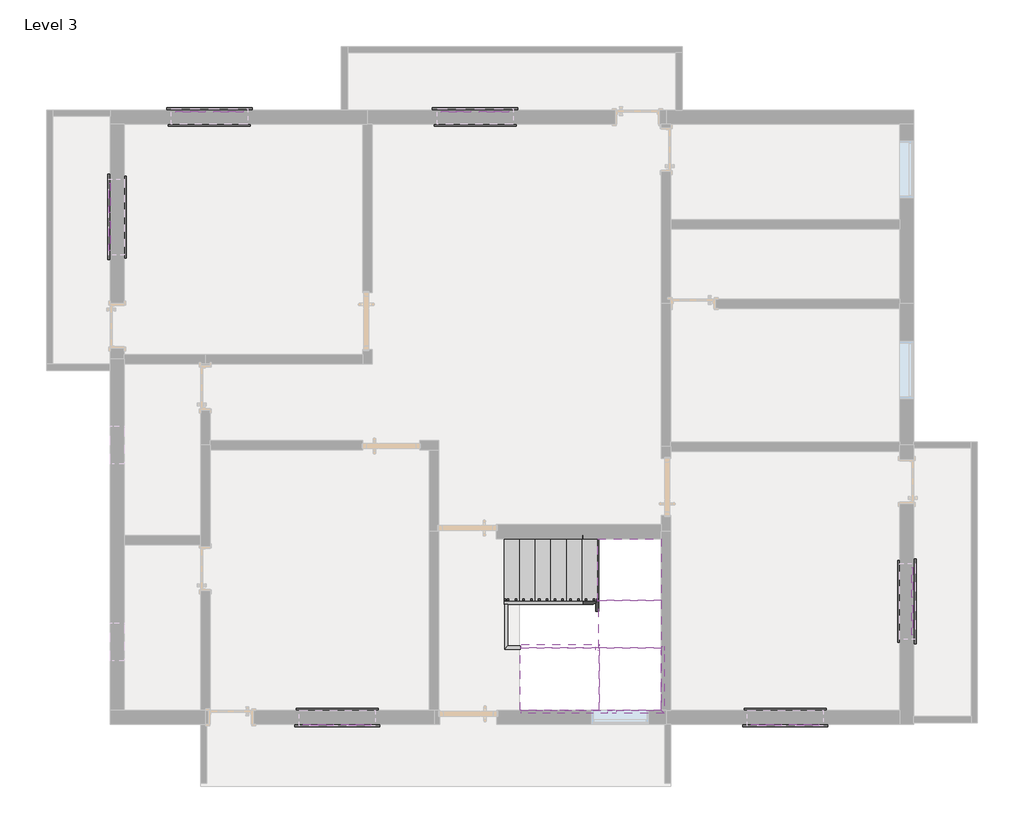
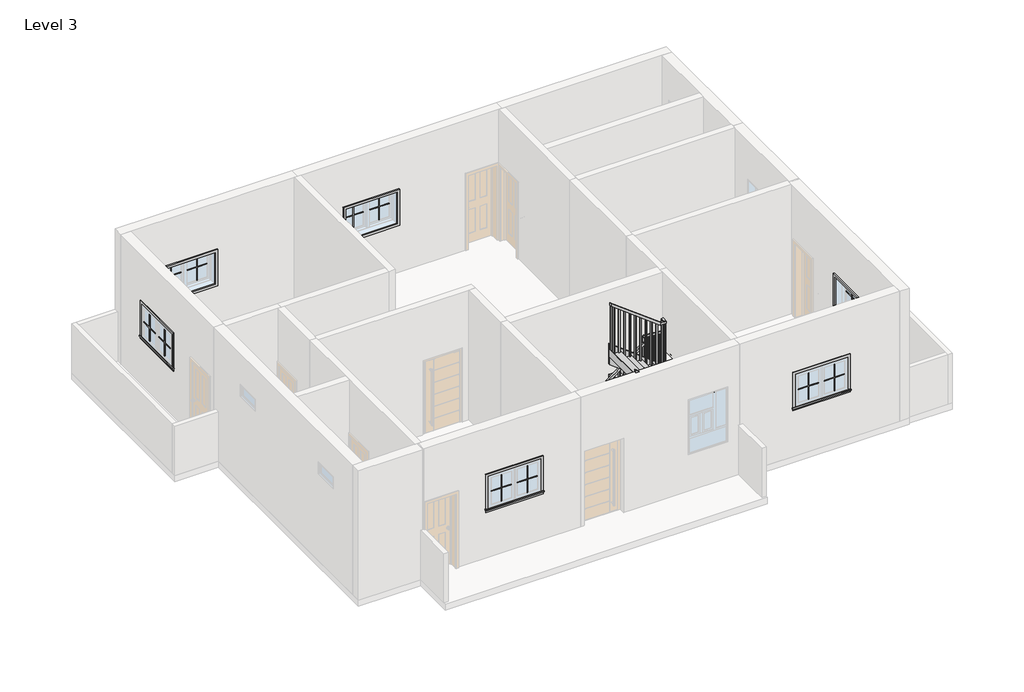
# One storey, part 3 of 3: 24 proxies, 11 members, 3 stair flights, 2 railings, 2 slabs.
"""IFC4 building model written with IfcOpenShell, lengths in millimetres."""

from ifc_helpers import new_model, si_unit, frame, origin, place, context, project, spatial, polyline, outline, extrude, faceted_brep, transform, mapped, element, save
from components import m_muntin_pattern_2x2_m_muntin_pattern_2x2_8d9e5da3, m_muntin_pattern_2x2_m_muntin_pattern_2x2_32a0f80e, m_trim_window_exterior_flat_with_sill_3a557199, m_trim_window_interior_flat_picture_frame_580345df, non_monolithic_landing_7cab632c, non_monolithic_landing_3909d1ad, stair_flight_50mm_tread_13mm_riser_c1773281, stair_flight_50mm_tread_13mm_riser_bd8d9b2e, stair_flight_50mm_tread_13mm_riser_69affff4

model = new_model("IFC4")

# Units and contexts
model_context = context("Model", 3, world=origin())
ifc_project = project(units=[si_unit("LENGTHUNIT", "METRE", prefix="MILLI")], contexts=[model_context])

# Site, building, storey
site = spatial("IfcSite", under=ifc_project)
building = spatial("IfcBuilding", under=site)
storey = spatial("IfcBuildingStorey", under=building, Name="Level 3", Elevation=6400.8)

# Proxies
placement = place(None, origin())
m_muntin_pattern_2x2_m_muntin_pattern_2x2_shape = m_muntin_pattern_2x2_m_muntin_pattern_2x2_8d9e5da3(model_context)
element("IfcBuildingElementProxy", 1, Name="M_Muntin Pattern_2x2 : M_Muntin Pattern_2x2", ObjectType="M_Muntin Pattern_2x2 : M_Muntin Pattern_2x2", at=placement, inside=storey, context=model_context, shape_type="MappedRepresentation", body=[
    mapped(m_muntin_pattern_2x2_m_muntin_pattern_2x2_shape, transform((-14356.7669909, -4470.2368509, 7689.85), x_axis=(-1.0, 0.0, 0.0), y_axis=(0.0, -1.0, 0.0), z_axis=(0.0, 0.0, 1.0))),
])
element("IfcBuildingElementProxy", 2, Name="M_Muntin Pattern_2x2 : M_Muntin Pattern_2x2", ObjectType="M_Muntin Pattern_2x2 : M_Muntin Pattern_2x2", at=placement, inside=storey, context=model_context, shape_type="MappedRepresentation", body=[
    mapped(m_muntin_pattern_2x2_m_muntin_pattern_2x2_shape, transform((-17007.0919909, 5340.5131491, 7689.85), x_axis=(1.0, 0.0, 0.0), y_axis=(0.0, 1.0, 0.0), z_axis=(0.0, 0.0, 1.0))),
])
element("IfcBuildingElementProxy", 3, Name="M_Muntin Pattern_2x2 : M_Muntin Pattern_2x2", ObjectType="M_Muntin Pattern_2x2 : M_Muntin Pattern_2x2", at=placement, inside=storey, context=model_context, shape_type="MappedRepresentation", body=[
    mapped(m_muntin_pattern_2x2_m_muntin_pattern_2x2_shape, transform((-18281.8544909, 3334.7006491, 7689.85), x_axis=(0.0, 1.0, 0.0), y_axis=(-1.0, 0.0, 0.0), z_axis=(0.0, 0.0, 1.0))),
])
element("IfcBuildingElementProxy", 4, Name="M_Muntin Pattern_2x2 : M_Muntin Pattern_2x2", ObjectType="M_Muntin Pattern_2x2 : M_Muntin Pattern_2x2", at=placement, inside=storey, context=model_context, shape_type="MappedRepresentation", body=[
    mapped(m_muntin_pattern_2x2_m_muntin_pattern_2x2_shape, transform((-12757.3544909, 5340.5131491, 7689.85), x_axis=(1.0, 0.0, 0.0), y_axis=(0.0, 1.0, 0.0), z_axis=(0.0, 0.0, 1.0))),
])
element("IfcBuildingElementProxy", 5, Name="M_Muntin Pattern_2x2 : M_Muntin Pattern_2x2", ObjectType="M_Muntin Pattern_2x2 : M_Muntin Pattern_2x2", at=placement, inside=storey, context=model_context, shape_type="MappedRepresentation", body=[
    mapped(m_muntin_pattern_2x2_m_muntin_pattern_2x2_shape, transform((-5448.5044909, -2207.2493509, 7689.85), x_axis=(0.0, -1.0, 0.0), y_axis=(1.0, 0.0, 0.0), z_axis=(0.0, 0.0, 1.0))),
])
element("IfcBuildingElementProxy", 6, Name="M_Muntin Pattern_2x2 : M_Muntin Pattern_2x2", ObjectType="M_Muntin Pattern_2x2 : M_Muntin Pattern_2x2", at=placement, inside=storey, context=model_context, shape_type="MappedRepresentation", body=[
    mapped(m_muntin_pattern_2x2_m_muntin_pattern_2x2_shape, transform((-7193.1669909, -4470.2368509, 7689.85), x_axis=(-1.0, 0.0, 0.0), y_axis=(0.0, -1.0, 0.0), z_axis=(0.0, 0.0, 1.0))),
])
m_muntin_pattern_2x2_m_muntin_pattern_2x2_2_shape = m_muntin_pattern_2x2_m_muntin_pattern_2x2_32a0f80e(model_context)
element("IfcBuildingElementProxy", 7, Name="M_Muntin Pattern_2x2 : M_Muntin Pattern_2x2", ObjectType="M_Muntin Pattern_2x2 : M_Muntin Pattern_2x2", at=placement, inside=storey, context=model_context, shape_type="MappedRepresentation", body=[
    mapped(m_muntin_pattern_2x2_m_muntin_pattern_2x2_2_shape, transform((-14963.1919909, -4470.2368509, 7689.85), x_axis=(1.0, 0.0, 0.0), y_axis=(0.0, 1.0, 0.0), z_axis=(0.0, 0.0, 1.0))),
])
element("IfcBuildingElementProxy", 8, Name="M_Muntin Pattern_2x2 : M_Muntin Pattern_2x2", ObjectType="M_Muntin Pattern_2x2 : M_Muntin Pattern_2x2", at=placement, inside=storey, context=model_context, shape_type="MappedRepresentation", body=[
    mapped(m_muntin_pattern_2x2_m_muntin_pattern_2x2_2_shape, transform((-16400.6669909, 5340.5131491, 7689.85), x_axis=(-1.0, 0.0, 0.0), y_axis=(0.0, -1.0, 0.0), z_axis=(0.0, 0.0, 1.0))),
])
element("IfcBuildingElementProxy", 9, Name="M_Muntin Pattern_2x2 : M_Muntin Pattern_2x2", ObjectType="M_Muntin Pattern_2x2 : M_Muntin Pattern_2x2", at=placement, inside=storey, context=model_context, shape_type="MappedRepresentation", body=[
    mapped(m_muntin_pattern_2x2_m_muntin_pattern_2x2_2_shape, transform((-18281.8544909, 3941.1256491, 7689.85), x_axis=(0.0, -1.0, 0.0), y_axis=(1.0, 0.0, 0.0), z_axis=(0.0, 0.0, 1.0))),
])
element("IfcBuildingElementProxy", 10, Name="M_Muntin Pattern_2x2 : M_Muntin Pattern_2x2", ObjectType="M_Muntin Pattern_2x2 : M_Muntin Pattern_2x2", at=placement, inside=storey, context=model_context, shape_type="MappedRepresentation", body=[
    mapped(m_muntin_pattern_2x2_m_muntin_pattern_2x2_2_shape, transform((-12150.9294909, 5340.5131491, 7689.85), x_axis=(-1.0, 0.0, 0.0), y_axis=(0.0, -1.0, 0.0), z_axis=(0.0, 0.0, 1.0))),
])
element("IfcBuildingElementProxy", 11, Name="M_Muntin Pattern_2x2 : M_Muntin Pattern_2x2", ObjectType="M_Muntin Pattern_2x2 : M_Muntin Pattern_2x2", at=placement, inside=storey, context=model_context, shape_type="MappedRepresentation", body=[
    mapped(m_muntin_pattern_2x2_m_muntin_pattern_2x2_2_shape, transform((-5448.5044909, -2813.6743509, 7689.85), x_axis=(0.0, 1.0, 0.0), y_axis=(-1.0, 0.0, 0.0), z_axis=(0.0, 0.0, 1.0))),
])
element("IfcBuildingElementProxy", 12, Name="M_Muntin Pattern_2x2 : M_Muntin Pattern_2x2", ObjectType="M_Muntin Pattern_2x2 : M_Muntin Pattern_2x2", at=placement, inside=storey, context=model_context, shape_type="MappedRepresentation", body=[
    mapped(m_muntin_pattern_2x2_m_muntin_pattern_2x2_2_shape, transform((-7799.5919909, -4470.2368509, 7689.85), x_axis=(1.0, 0.0, 0.0), y_axis=(0.0, 1.0, 0.0), z_axis=(0.0, 0.0, 1.0))),
])
m_trim_window_exterior_flat_with_sill_shape = m_trim_window_exterior_flat_with_sill_3a557199(model_context)
element("IfcBuildingElementProxy", 13, Name="M_Trim-Window-Exterior-Flat : with Sill", ObjectType="M_Trim-Window-Exterior-Flat : with Sill", at=placement, inside=storey, context=model_context, shape_type="MappedRepresentation", body=[
    mapped(m_trim_window_exterior_flat_with_sill_shape, transform((-14659.9794909, -4479.7618509, 8420.0), x_axis=(1.0, 0.0, 0.0), y_axis=(0.0, 0.0, 1.0), z_axis=(0.0, -1.0, 0.0))),
])
element("IfcBuildingElementProxy", 14, Name="M_Trim-Window-Exterior-Flat : with Sill", ObjectType="M_Trim-Window-Exterior-Flat : with Sill", at=placement, inside=storey, context=model_context, shape_type="MappedRepresentation", body=[
    mapped(m_trim_window_exterior_flat_with_sill_shape, transform((-16703.8794909, 5350.0381491, 8420.0), x_axis=(-1.0, 0.0, 0.0), y_axis=(0.0, 0.0, 1.0), z_axis=(0.0, 1.0, 0.0))),
])
element("IfcBuildingElementProxy", 15, Name="M_Trim-Window-Exterior-Flat : with Sill", ObjectType="M_Trim-Window-Exterior-Flat : with Sill", at=placement, inside=storey, context=model_context, shape_type="MappedRepresentation", body=[
    mapped(m_trim_window_exterior_flat_with_sill_shape, transform((-18291.3794909, 3637.9131491, 8420.0), x_axis=(0.0, -1.0, 0.0), y_axis=(0.0, 0.0, 1.0), z_axis=(-1.0, 0.0, 0.0))),
])
element("IfcBuildingElementProxy", 16, Name="M_Trim-Window-Exterior-Flat : with Sill", ObjectType="M_Trim-Window-Exterior-Flat : with Sill", at=placement, inside=storey, context=model_context, shape_type="MappedRepresentation", body=[
    mapped(m_trim_window_exterior_flat_with_sill_shape, transform((-12454.1419909, 5350.0381491, 8420.0), x_axis=(-1.0, 0.0, 0.0), y_axis=(0.0, 0.0, 1.0), z_axis=(0.0, 1.0, 0.0))),
])
element("IfcBuildingElementProxy", 17, Name="M_Trim-Window-Exterior-Flat : with Sill", ObjectType="M_Trim-Window-Exterior-Flat : with Sill", at=placement, inside=storey, context=model_context, shape_type="MappedRepresentation", body=[
    mapped(m_trim_window_exterior_flat_with_sill_shape, transform((-5438.9794909, -2510.4618509, 8420.0), x_axis=(0.0, 1.0, 0.0), y_axis=(0.0, 0.0, 1.0), z_axis=(1.0, 0.0, 0.0))),
])
element("IfcBuildingElementProxy", 18, Name="M_Trim-Window-Exterior-Flat : with Sill", ObjectType="M_Trim-Window-Exterior-Flat : with Sill", at=placement, inside=storey, context=model_context, shape_type="MappedRepresentation", body=[
    mapped(m_trim_window_exterior_flat_with_sill_shape, transform((-7496.3794909, -4479.7618509, 8420.0), x_axis=(1.0, 0.0, 0.0), y_axis=(0.0, 0.0, 1.0), z_axis=(0.0, -1.0, 0.0))),
])
m_trim_window_interior_flat_picture_frame_shape = m_trim_window_interior_flat_picture_frame_580345df(model_context)
element("IfcBuildingElementProxy", 19, Name="M_Trim-Window-Interior-Flat : Picture Frame", ObjectType="M_Trim-Window-Interior-Flat : Picture Frame", at=placement, inside=storey, context=model_context, shape_type="MappedRepresentation", body=[
    mapped(m_trim_window_interior_flat_picture_frame_shape, transform((-14659.9794909, -4251.1618509, 8420.0), x_axis=(-1.0, 0.0, 0.0), y_axis=(0.0, 0.0, 1.0), z_axis=(0.0, 1.0, 0.0))),
])
element("IfcBuildingElementProxy", 20, Name="M_Trim-Window-Interior-Flat : Picture Frame", ObjectType="M_Trim-Window-Interior-Flat : Picture Frame", at=placement, inside=storey, context=model_context, shape_type="MappedRepresentation", body=[
    mapped(m_trim_window_interior_flat_picture_frame_shape, transform((-16703.8794909, 5121.4381491, 8420.0), x_axis=(1.0, 0.0, 0.0), y_axis=(0.0, 0.0, 1.0), z_axis=(0.0, -1.0, 0.0))),
])
element("IfcBuildingElementProxy", 21, Name="M_Trim-Window-Interior-Flat : Picture Frame", ObjectType="M_Trim-Window-Interior-Flat : Picture Frame", at=placement, inside=storey, context=model_context, shape_type="MappedRepresentation", body=[
    mapped(m_trim_window_interior_flat_picture_frame_shape, transform((-18062.7794909, 3637.9131491, 8420.0), x_axis=(0.0, 1.0, 0.0), y_axis=(0.0, 0.0, 1.0), z_axis=(1.0, 0.0, 0.0))),
])
element("IfcBuildingElementProxy", 22, Name="M_Trim-Window-Interior-Flat : Picture Frame", ObjectType="M_Trim-Window-Interior-Flat : Picture Frame", at=placement, inside=storey, context=model_context, shape_type="MappedRepresentation", body=[
    mapped(m_trim_window_interior_flat_picture_frame_shape, transform((-12454.1419909, 5121.4381491, 8420.0), x_axis=(1.0, 0.0, 0.0), y_axis=(0.0, 0.0, 1.0), z_axis=(0.0, -1.0, 0.0))),
])
element("IfcBuildingElementProxy", 23, Name="M_Trim-Window-Interior-Flat : Picture Frame", ObjectType="M_Trim-Window-Interior-Flat : Picture Frame", at=placement, inside=storey, context=model_context, shape_type="MappedRepresentation", body=[
    mapped(m_trim_window_interior_flat_picture_frame_shape, transform((-5667.5794909, -2510.4618509, 8420.0), x_axis=(0.0, -1.0, 0.0), y_axis=(0.0, 0.0, 1.0), z_axis=(-1.0, 0.0, 0.0))),
])
element("IfcBuildingElementProxy", 24, Name="M_Trim-Window-Interior-Flat : Picture Frame", ObjectType="M_Trim-Window-Interior-Flat : Picture Frame", at=placement, inside=storey, context=model_context, shape_type="MappedRepresentation", body=[
    mapped(m_trim_window_interior_flat_picture_frame_shape, transform((-7496.3794909, -4251.1618509, 8420.0), x_axis=(-1.0, 0.0, 0.0), y_axis=(0.0, 0.0, 1.0), z_axis=(0.0, 1.0, 0.0))),
])

# Members
element("IfcMember", 25, ObjectType="Stringer - 50mm Width", at=placement, inside=storey, context=model_context, shape_type="SweptSolid", body=[
    extrude(outline(polyline([(6654.3429417, -11992.1794909), (6400.8, -11992.1794909), (6400.8, -11663.9259909), (7368.6117647, -10378.7116427), (7768.6117647, -10512.4761733), (6654.3429417, -11992.1794909)])), frame((0.0, -1507.9618509, 0.0), z_axis=(0.0, 1.0, 0.0), x_axis=(0.0, 0.0, 1.0)), (0.0, 0.0, 1.0), 50.0),
])
element("IfcMember", 26, ObjectType="Stringer - 50mm Width", at=placement, inside=storey, context=model_context, shape_type="Brep", body=[
    faceted_brep([(-11992.1794909, -2557.9876321, 6400.8), (-11992.1794909, -2507.9876321, 6400.8), (-11663.9259909, -2507.9876321, 6400.8), (-11663.9259909, -2557.9876321, 6400.8), (-11992.1794909, -2557.9876321, 6654.3429417), (-10569.4898929, -2557.9876321, 7224.949009), (-10569.4898929, -2557.9876321, 7725.6784216), (-10492.1794909, -2507.9876321, 7283.1664703), (-10492.1794909, -2507.9876321, 7768.6117647), (-10512.4761733, -2521.1143795, 7768.6117647), (-11992.1794909, -2507.9876321, 6654.3429417), (-10512.4761733, -2507.9876321, 7768.6117647)], [[[0, 1, 2, 3]], [[4, 0, 3, 5, 6]], [[6, 5, 7, 8, 9]], [[2, 7, 5, 3]], [[1, 10, 11, 8, 7, 2]], [[11, 9, 8]], [[10, 4, 6, 9, 11]], [[4, 10, 1, 0]]]),
])
element("IfcMember", 27, ObjectType="Stringer - 50mm Width", at=placement, inside=storey, context=model_context, shape_type="SweptSolid", body=[
    extrude(outline(polyline([(-2228.2651685, 7768.6117647), (-2362.029699, 7368.6117647), (-3362.029699, 8121.6470588), (-3228.2651685, 8521.6470588), (-2228.2651685, 7768.6117647)])), frame((-9477.5794909, 0.0, 0.0), z_axis=(1.0, 0.0, 0.0), x_axis=(0.0, 1.0, 0.0)), (0.0, 0.0, 1.0), 50.0),
])
element("IfcMember", 28, ObjectType="Stringer - 50mm Width", at=placement, inside=storey, context=model_context, shape_type="Brep", body=[
    faceted_brep([(-10527.6052721, -3234.9066499, 8521.6470588), (-10527.6052721, -3234.9066499, 8025.9189161), (-10477.6052721, -3248.5618509, 8036.2017644), (-10477.6052721, -3248.5618509, 8521.6470588), (-10477.6052721, -3228.2651685, 8521.6470588), (-10527.6052721, -3228.2651685, 8521.6470588), (-10477.6052721, -2498.5618509, 7972.1547064), (-10527.6052721, -2530.8990259, 7996.5057405), (-10477.6052721, -2498.5618509, 7471.4252938), (-10527.6052721, -2530.8990259, 7495.7763279)], [[[0, 1, 2, 3]], [[4, 5, 0, 3]], [[6, 7, 5, 4]], [[7, 6, 8, 9]], [[7, 9, 1, 0, 5]], [[8, 6, 4, 3, 2]], [[9, 8, 2, 1]]]),
])
element("IfcMember", 29, ObjectType="Stringer - 50mm Width", at=placement, inside=storey, context=model_context, shape_type="Brep", body=[
    faceted_brep([(-9477.5794909, -2228.2651685, 7768.6117647), (-9427.5794909, -2228.2651685, 7768.6117647), (-9427.5794909, -1457.9618509, 7768.6117647), (-9477.5794909, -1507.9618509, 7768.6117647), (-9477.5794909, -2362.029699, 7368.6117647), (-9477.5794909, -1507.9618509, 7368.6117647), (-9427.5794909, -2362.029699, 7368.6117647), (-9427.5794909, -1457.9618509, 7368.6117647)], [[[0, 1, 2, 3]], [[4, 0, 3, 5]], [[6, 4, 5, 7]], [[1, 6, 7, 2]], [[1, 0, 4, 6]], [[2, 7, 5, 3]]]),
])
element("IfcMember", 30, ObjectType="Stringer - 50mm Width", at=placement, inside=storey, context=model_context, shape_type="Brep", body=[
    faceted_brep([(-9477.5794909, -1507.9618509, 7768.6117647), (-9427.5794909, -1457.9618509, 7768.6117647), (-10512.4761733, -1457.9618509, 7768.6117647), (-10512.4761733, -1507.9618509, 7768.6117647), (-9477.5794909, -1507.9618509, 7368.6117647), (-10378.7116427, -1507.9618509, 7368.6117647), (-9427.5794909, -1457.9618509, 7368.6117647), (-10378.7116427, -1457.9618509, 7368.6117647)], [[[0, 1, 2, 3]], [[4, 0, 3, 5]], [[6, 4, 5, 7]], [[1, 6, 7, 2]], [[1, 0, 4, 6]], [[2, 7, 5, 3]]]),
])
element("IfcMember", 31, ObjectType="Stringer - 50mm Width", at=placement, inside=storey, context=model_context, shape_type="SweptSolid", body=[
    extrude(outline(polyline([(8121.6470588, -10331.6473391), (8521.6470588, -10197.8828085), (9666.4841182, -11718.1794909), (9165.7547056, -11718.1794909), (8121.6470588, -10331.6473391)])), frame((0.0, -4301.1618509, 0.0), z_axis=(0.0, 1.0, 0.0), x_axis=(0.0, 0.0, 1.0)), (0.0, 0.0, 1.0), 50.0),
])
element("IfcMember", 32, ObjectType="Stringer - 50mm Width", at=placement, inside=storey, context=model_context, shape_type="SweptSolid", body=[
    extrude(outline(polyline([(8224.4605879, -10468.1794909), (8725.1900005, -10468.1794909), (9666.4841182, -11718.1794909), (9165.7547056, -11718.1794909), (8224.4605879, -10468.1794909)])), frame((0.0, -3251.1360696, 0.0), z_axis=(0.0, 1.0, 0.0), x_axis=(0.0, 0.0, 1.0)), (0.0, 0.0, 1.0), 50.0),
])
element("IfcMember", 33, ObjectType="Stringer - 50mm Width", at=placement, inside=storey, context=model_context, shape_type="Brep", body=[
    faceted_brep([(-10197.8828085, -4251.1618509, 8521.6470588), (-10197.8828085, -4301.1618509, 8521.6470588), (-9427.5794909, -4301.1618509, 8521.6470588), (-9477.5794909, -4251.1618509, 8521.6470588), (-10331.6473391, -4251.1618509, 8121.6470588), (-9477.5794909, -4251.1618509, 8121.6470588), (-10331.6473391, -4301.1618509, 8121.6470588), (-9427.5794909, -4301.1618509, 8121.6470588)], [[[0, 1, 2, 3]], [[4, 0, 3, 5]], [[6, 4, 5, 7]], [[1, 6, 7, 2]], [[1, 0, 4, 6]], [[2, 7, 5, 3]]]),
])
element("IfcMember", 34, ObjectType="Stringer - 50mm Width", at=placement, inside=storey, context=model_context, shape_type="Brep", body=[
    faceted_brep([(-9477.5794909, -4251.1618509, 8521.6470588), (-9427.5794909, -4301.1618509, 8521.6470588), (-9427.5794909, -3228.2651685, 8521.6470588), (-9477.5794909, -3228.2651685, 8521.6470588), (-9477.5794909, -4251.1618509, 8121.6470588), (-9477.5794909, -3362.029699, 8121.6470588), (-9427.5794909, -4301.1618509, 8121.6470588), (-9427.5794909, -3362.029699, 8121.6470588)], [[[0, 1, 2, 3]], [[4, 0, 3, 5]], [[6, 4, 5, 7]], [[1, 6, 7, 2]], [[1, 0, 4, 6]], [[2, 7, 5, 3]]]),
])
element("IfcMember", 35, ObjectType="Stringer - 50mm Width", at=placement, inside=storey, context=model_context, shape_type="SweptSolid", body=[
    extrude(outline(polyline([(-10527.6052721, -3286.7377652), (-10527.6052721, -3234.9066499), (-10468.1794909, -3251.1360696), (-10468.1794909, -3302.9671849), (-10527.6052721, -3286.7377652)])), frame((0.0, 0.0, 8121.6470588), z_axis=(0.0, 0.0, 1.0), x_axis=(1.0, 0.0, 0.0)), (0.0, 0.0, 1.0), 400.0),
])

# Railings
element("IfcRailing", 36, ObjectType="1100mm", at=placement, inside=storey, context=model_context, shape_type="SolidModel", body=[
    faceted_brep([(-11992.1794909, -2457.5876321, 7689.0588235), (-11992.1794909, -2457.5876321, 7626.467647), (-11992.1794909, -2507.5876321, 7626.467647), (-11992.1794909, -2507.5876321, 7689.0588235), (-10506.1686883, -2457.5876321, 8808.0774053), (-10493.1861187, -2507.5876321, 8817.8537384), (-10475.1839648, -2507.5876321, 8768.8188191), (-10488.1665344, -2457.5876321, 8759.042486)], [[[0, 1, 2, 3]], [[4, 5, 6, 7]], [[1, 0, 4, 7]], [[2, 1, 7, 6]], [[3, 2, 6, 5]], [[0, 3, 5, 4]]]),
    faceted_brep([(-10507.8033465, -2458.0701724, 8818.6117647), (-10492.6871017, -2448.2938394, 8768.6117647), (-10476.4352157, -2497.3287587, 8768.6117647), (-10491.5514605, -2507.1050918, 8818.6117647), (-10486.7741604, -2444.469683, 8818.6117647), (-10459.6209288, -2486.4542279, 8818.6117647), (-10417.6363839, -2459.3009964, 8768.6117647), (-10444.7896154, -2417.3164514, 8768.6117647)], [[[0, 1, 2, 3]], [[4, 5, 6, 7]], [[1, 0, 4, 7]], [[2, 1, 7, 6]], [[3, 2, 6, 5]], [[0, 3, 5, 4]]]),
    faceted_brep([(-10486.7741604, -2444.469683, 8818.6117647), (-10444.7896154, -2417.3164514, 8768.6117647), (-10417.6363839, -2459.3009964, 8768.6117647), (-10459.6209288, -2486.4542279, 8818.6117647), (-10486.7741604, -2444.469683, 8944.124782), (-10459.6209288, -2486.4542279, 8923.1833848), (-10417.6363839, -2459.3009964, 8936.7270973), (-10444.7896154, -2417.3164514, 8957.6684945)], [[[0, 1, 2, 3]], [[4, 5, 6, 7]], [[1, 0, 4, 7]], [[2, 1, 7, 6]], [[3, 2, 6, 5]], [[0, 3, 5, 4]]]),
    faceted_brep([(-10427.2052721, -2426.8853397, 8952.8956456), (-10427.2052721, -2476.8853397, 8927.9562337), (-10477.2052721, -2476.8853397, 8927.9562337), (-10477.2052721, -2426.8853397, 8952.8956456), (-10427.2052721, -3176.5360696, 9517.4091035), (-10427.2052721, -3226.5360696, 9492.4696916), (-10477.2052721, -3226.5360696, 9492.4696916), (-10477.2052721, -3176.5360696, 9517.4091035), (-10427.2052721, -3176.5360696, 9823.1802613), (-10427.2052721, -3226.5360696, 9773.1802613), (-10477.2052721, -3226.5360696, 9773.1802613), (-10477.2052721, -3176.5360696, 9823.1802613), (-10427.2052721, -3301.5360696, 9823.1802613), (-10427.2052721, -3301.5360696, 9773.1802613), (-10477.2052721, -3251.5360696, 9773.1802613), (-10477.2052721, -3251.5360696, 9823.1802613), (-10552.2052721, -3301.5360696, 9823.1802613), (-10568.9258385, -3301.5360696, 9773.1802613), (-10568.9258385, -3251.5360696, 9773.1802613), (-10552.2052721, -3251.5360696, 9823.1802613), (-11718.1794909, -3301.5360696, 10701.2), (-11718.1794909, -3251.5360696, 10701.2), (-11718.1794909, -3251.5360696, 10638.6088234), (-11718.1794909, -3301.5360696, 10638.6088234)], [[[0, 1, 2, 3]], [[1, 0, 4, 5]], [[2, 1, 5, 6]], [[3, 2, 6, 7]], [[0, 3, 7, 4]], [[5, 4, 8, 9]], [[6, 5, 9, 10]], [[7, 6, 10, 11]], [[4, 7, 11, 8]], [[9, 8, 12, 13]], [[10, 9, 13, 14]], [[11, 10, 14, 15]], [[8, 11, 15, 12]], [[13, 12, 16, 17]], [[14, 13, 17, 18]], [[15, 14, 18, 19]], [[12, 15, 19, 16]], [[20, 21, 22, 23]], [[17, 16, 20, 23]], [[18, 17, 23, 22]], [[19, 18, 22, 21]], [[16, 19, 21, 20]]]),
    extrude(outline(polyline([(9412.9411765, -11627.2052721), (10570.1020258, -11627.2052721), (10588.9279082, -11652.2052721), (9412.9411765, -11652.2052721), (9412.9411765, -11627.2052721)])), frame((0.0, -3289.0360696, 0.0), z_axis=(0.0, 1.0, 0.0), x_axis=(0.0, 0.0, 1.0)), (0.0, 0.0, 1.0), 25.0),
    extrude(outline(polyline([(9412.9411765, -11502.2052721), (10475.9726141, -11502.2052721), (10494.7984964, -11527.2052721), (9412.9411765, -11527.2052721), (9412.9411765, -11502.2052721)])), frame((0.0, -3289.0360696, 0.0), z_axis=(0.0, 1.0, 0.0), x_axis=(0.0, 0.0, 1.0)), (0.0, 0.0, 1.0), 25.0),
    extrude(outline(polyline([(9224.6823529, -11377.2052721), (10381.8432023, -11377.2052721), (10400.6690847, -11402.2052721), (9224.6823529, -11402.2052721), (9224.6823529, -11377.2052721)])), frame((0.0, -3289.0360696, 0.0), z_axis=(0.0, 1.0, 0.0), x_axis=(0.0, 0.0, 1.0)), (0.0, 0.0, 1.0), 25.0),
    extrude(outline(polyline([(9224.6823529, -11252.2052721), (10287.7137906, -11252.2052721), (10306.5396729, -11277.2052721), (9224.6823529, -11277.2052721), (9224.6823529, -11252.2052721)])), frame((0.0, -3289.0360696, 0.0), z_axis=(0.0, 1.0, 0.0), x_axis=(0.0, 0.0, 1.0)), (0.0, 0.0, 1.0), 25.0),
    extrude(outline(polyline([(9036.4235294, -11127.2052721), (10193.5843788, -11127.2052721), (10212.4102611, -11152.2052721), (9036.4235294, -11152.2052721), (9036.4235294, -11127.2052721)])), frame((0.0, -3289.0360696, 0.0), z_axis=(0.0, 1.0, 0.0), x_axis=(0.0, 0.0, 1.0)), (0.0, 0.0, 1.0), 25.0),
    extrude(outline(polyline([(9036.4235294, -11002.2052721), (10099.454967, -11002.2052721), (10118.2808494, -11027.2052721), (9036.4235294, -11027.2052721), (9036.4235294, -11002.2052721)])), frame((0.0, -3289.0360696, 0.0), z_axis=(0.0, 1.0, 0.0), x_axis=(0.0, 0.0, 1.0)), (0.0, 0.0, 1.0), 25.0),
    extrude(outline(polyline([(8848.1647059, -10877.2052721), (10005.3255553, -10877.2052721), (10024.1514376, -10902.2052721), (8848.1647059, -10902.2052721), (8848.1647059, -10877.2052721)])), frame((0.0, -3289.0360696, 0.0), z_axis=(0.0, 1.0, 0.0), x_axis=(0.0, 0.0, 1.0)), (0.0, 0.0, 1.0), 25.0),
    extrude(outline(polyline([(8848.1647059, -10752.2052721), (9911.1961435, -10752.2052721), (9930.0220258, -10777.2052721), (8848.1647059, -10777.2052721), (8848.1647059, -10752.2052721)])), frame((0.0, -3289.0360696, 0.0), z_axis=(0.0, 1.0, 0.0), x_axis=(0.0, 0.0, 1.0)), (0.0, 0.0, 1.0), 25.0),
    extrude(outline(polyline([(8659.9058824, -10627.2052721), (9817.0667317, -10627.2052721), (9835.8926141, -10652.2052721), (8659.9058824, -10652.2052721), (8659.9058824, -10627.2052721)])), frame((0.0, -3289.0360696, 0.0), z_axis=(0.0, 1.0, 0.0), x_axis=(0.0, 0.0, 1.0)), (0.0, 0.0, 1.0), 25.0),
    extrude(outline(polyline([(-10502.2052721, -3264.0360696), (-10502.2052721, -3289.0360696), (-10527.2052721, -3289.0360696), (-10527.2052721, -3264.0360696), (-10502.2052721, -3264.0360696)])), frame((0.0, 0.0, 8659.9058824), z_axis=(0.0, 0.0, 1.0), x_axis=(1.0, 0.0, 0.0)), (0.0, 0.0, 1.0), 1113.2743789),
    extrude(outline(polyline([(-10464.7052721, -3251.8853397), (-10439.7052721, -3251.8853397), (-10439.7052721, -3276.8853397), (-10464.7052721, -3276.8853397), (-10464.7052721, -3251.8853397)])), frame((0.0, 0.0, 8471.6470588), z_axis=(0.0, 0.0, 1.0), x_axis=(1.0, 0.0, 0.0)), (0.0, 0.0, 1.0), 1301.5332024),
    extrude(outline(polyline([(-3126.8853397, 9417.4291749), (-3126.8853397, 8283.3882353), (-3151.8853397, 8283.3882353), (-3151.8853397, 9436.2550572), (-3126.8853397, 9417.4291749)])), frame((-10464.7052721, 0.0, 0.0), z_axis=(1.0, 0.0, 0.0), x_axis=(0.0, 1.0, 0.0)), (0.0, 0.0, 1.0), 25.0),
    extrude(outline(polyline([(-3001.8853397, 9323.2997631), (-3001.8853397, 8283.3882353), (-3026.8853397, 8283.3882353), (-3026.8853397, 9342.1256455), (-3001.8853397, 9323.2997631)])), frame((-10464.7052721, 0.0, 0.0), z_axis=(1.0, 0.0, 0.0), x_axis=(0.0, 1.0, 0.0)), (0.0, 0.0, 1.0), 25.0),
    extrude(outline(polyline([(-2876.8853397, 9229.1703513), (-2876.8853397, 8095.1294118), (-2901.8853397, 8095.1294118), (-2901.8853397, 9247.9962337), (-2876.8853397, 9229.1703513)])), frame((-10464.7052721, 0.0, 0.0), z_axis=(1.0, 0.0, 0.0), x_axis=(0.0, 1.0, 0.0)), (0.0, 0.0, 1.0), 25.0),
    extrude(outline(polyline([(-2751.8853397, 9135.0409396), (-2751.8853397, 8095.1294118), (-2776.8853397, 8095.1294118), (-2776.8853397, 9153.8668219), (-2751.8853397, 9135.0409396)])), frame((-10464.7052721, 0.0, 0.0), z_axis=(1.0, 0.0, 0.0), x_axis=(0.0, 1.0, 0.0)), (0.0, 0.0, 1.0), 25.0),
    extrude(outline(polyline([(-2626.8853397, 9040.9115278), (-2626.8853397, 7906.8705882), (-2651.8853397, 7906.8705882), (-2651.8853397, 9059.7374102), (-2626.8853397, 9040.9115278)])), frame((-10464.7052721, 0.0, 0.0), z_axis=(1.0, 0.0, 0.0), x_axis=(0.0, 1.0, 0.0)), (0.0, 0.0, 1.0), 25.0),
    extrude(outline(polyline([(-2501.8853397, 8946.782116), (-2501.8853397, 7906.8705882), (-2526.8853397, 7906.8705882), (-2526.8853397, 8965.6079984), (-2501.8853397, 8946.782116)])), frame((-10464.7052721, 0.0, 0.0), z_axis=(1.0, 0.0, 0.0), x_axis=(0.0, 1.0, 0.0)), (0.0, 0.0, 1.0), 25.0),
    extrude(outline(polyline([(8699.5429411, -10567.1794909), (7530.3529412, -10567.1794909), (7530.3529412, -10542.1794909), (8718.3688234, -10542.1794909), (8699.5429411, -10567.1794909)])), frame((0.0, -2495.0876321, 0.0), z_axis=(0.0, 1.0, 0.0), x_axis=(0.0, 0.0, 1.0)), (0.0, 0.0, 1.0), 25.0),
    extrude(outline(polyline([(8605.4135293, -10692.1794909), (7530.3529412, -10692.1794909), (7530.3529412, -10667.1794909), (8624.2394117, -10667.1794909), (8605.4135293, -10692.1794909)])), frame((0.0, -2495.0876321, 0.0), z_axis=(0.0, 1.0, 0.0), x_axis=(0.0, 0.0, 1.0)), (0.0, 0.0, 1.0), 25.0),
    extrude(outline(polyline([(8511.2841175, -10817.1794909), (7342.0941176, -10817.1794909), (7342.0941176, -10792.1794909), (8530.1099999, -10792.1794909), (8511.2841175, -10817.1794909)])), frame((0.0, -2495.0876321, 0.0), z_axis=(0.0, 1.0, 0.0), x_axis=(0.0, 0.0, 1.0)), (0.0, 0.0, 1.0), 25.0),
    extrude(outline(polyline([(8417.1547058, -10942.1794909), (7342.0941176, -10942.1794909), (7342.0941176, -10917.1794909), (8435.9805881, -10917.1794909), (8417.1547058, -10942.1794909)])), frame((0.0, -2495.0876321, 0.0), z_axis=(0.0, 1.0, 0.0), x_axis=(0.0, 0.0, 1.0)), (0.0, 0.0, 1.0), 25.0),
    extrude(outline(polyline([(8323.025294, -11067.1794909), (7153.8352941, -11067.1794909), (7153.8352941, -11042.1794909), (8341.8511764, -11042.1794909), (8323.025294, -11067.1794909)])), frame((0.0, -2495.0876321, 0.0), z_axis=(0.0, 1.0, 0.0), x_axis=(0.0, 0.0, 1.0)), (0.0, 0.0, 1.0), 25.0),
    extrude(outline(polyline([(8228.8958822, -11192.1794909), (7153.8352941, -11192.1794909), (7153.8352941, -11167.1794909), (8247.7217646, -11167.1794909), (8228.8958822, -11192.1794909)])), frame((0.0, -2495.0876321, 0.0), z_axis=(0.0, 1.0, 0.0), x_axis=(0.0, 0.0, 1.0)), (0.0, 0.0, 1.0), 25.0),
    extrude(outline(polyline([(8134.7664705, -11317.1794909), (6965.5764706, -11317.1794909), (6965.5764706, -11292.1794909), (8153.5923528, -11292.1794909), (8134.7664705, -11317.1794909)])), frame((0.0, -2495.0876321, 0.0), z_axis=(0.0, 1.0, 0.0), x_axis=(0.0, 0.0, 1.0)), (0.0, 0.0, 1.0), 25.0),
    extrude(outline(polyline([(8040.6370587, -11442.1794909), (6965.5764706, -11442.1794909), (6965.5764706, -11417.1794909), (8059.4629411, -11417.1794909), (8040.6370587, -11442.1794909)])), frame((0.0, -2495.0876321, 0.0), z_axis=(0.0, 1.0, 0.0), x_axis=(0.0, 0.0, 1.0)), (0.0, 0.0, 1.0), 25.0),
    extrude(outline(polyline([(7946.507647, -11567.1794909), (6777.3176471, -11567.1794909), (6777.3176471, -11542.1794909), (7965.3335293, -11542.1794909), (7946.507647, -11567.1794909)])), frame((0.0, -2495.0876321, 0.0), z_axis=(0.0, 1.0, 0.0), x_axis=(0.0, 0.0, 1.0)), (0.0, 0.0, 1.0), 25.0),
    extrude(outline(polyline([(7852.3782352, -11692.1794909), (6777.3176471, -11692.1794909), (6777.3176471, -11667.1794909), (7871.2041175, -11667.1794909), (7852.3782352, -11692.1794909)])), frame((0.0, -2495.0876321, 0.0), z_axis=(0.0, 1.0, 0.0), x_axis=(0.0, 0.0, 1.0)), (0.0, 0.0, 1.0), 25.0),
    extrude(outline(polyline([(7758.2488234, -11817.1794909), (6589.0588235, -11817.1794909), (6589.0588235, -11792.1794909), (7777.0747058, -11792.1794909), (7758.2488234, -11817.1794909)])), frame((0.0, -2495.0876321, 0.0), z_axis=(0.0, 1.0, 0.0), x_axis=(0.0, 0.0, 1.0)), (0.0, 0.0, 1.0), 25.0),
    extrude(outline(polyline([(7664.1194117, -11942.1794909), (6589.0588235, -11942.1794909), (6589.0588235, -11917.1794909), (7682.945294, -11917.1794909), (7664.1194117, -11942.1794909)])), frame((0.0, -2495.0876321, 0.0), z_axis=(0.0, 1.0, 0.0), x_axis=(0.0, 0.0, 1.0)), (0.0, 0.0, 1.0), 25.0),
    extrude(outline(polyline([(-10464.7052721, -3264.0360696), (-10439.7052721, -3264.0360696), (-10439.7052721, -3289.0360696), (-10464.7052721, -3289.0360696), (-10464.7052721, -3264.0360696)])), frame((0.0, 0.0, 8471.6470588), z_axis=(0.0, 0.0, 1.0), x_axis=(1.0, 0.0, 0.0)), (0.0, 0.0, 1.0), 1301.5332024),
    extrude(outline(polyline([(-10455.9131005, -2469.1697838), (-10469.4897163, -2448.1775113), (-10448.4974438, -2434.6008955), (-10434.920828, -2455.593168), (-10455.9131005, -2469.1697838)])), frame((0.0, 0.0, 7718.6117647), z_axis=(0.0, 0.0, 1.0), x_axis=(1.0, 0.0, 0.0)), (0.0, 0.0, 1.0), 1050.0),
    extrude(outline(polyline([(8740.9614541, -10512.1774035), (7530.3529412, -10512.1774035), (7530.3529412, -10487.1774035), (8759.7873365, -10487.1774035), (8740.9614541, -10512.1774035)])), frame((0.0, -2495.0876321, 0.0), z_axis=(0.0, 1.0, 0.0), x_axis=(0.0, 0.0, 1.0)), (0.0, 0.0, 1.0), 25.0),
    extrude(outline(polyline([(9412.9411765, -11693.1794909), (10619.7829411, -11693.1794909), (10638.6088234, -11718.1794909), (9412.9411765, -11718.1794909), (9412.9411765, -11693.1794909)])), frame((0.0, -3289.0360696, 0.0), z_axis=(0.0, 1.0, 0.0), x_axis=(0.0, 0.0, 1.0)), (0.0, 0.0, 1.0), 25.0),
    extrude(outline(polyline([(7626.467647, -11992.1794909), (6589.0588235, -11992.1794909), (6589.0588235, -11967.1794909), (7645.2935293, -11967.1794909), (7626.467647, -11992.1794909)])), frame((0.0, -2495.0876321, 0.0), z_axis=(0.0, 1.0, 0.0), x_axis=(0.0, 0.0, 1.0)), (0.0, 0.0, 1.0), 25.0),
])
element("IfcRailing", 37, ObjectType="900mm", at=placement, inside=storey, context=model_context, shape_type="SolidModel", body=[
    faceted_brep([(-11730.6794909, -3276.1360696, 7442.2), (-11730.6794909, -3276.1360696, 7392.2), (-11730.6794909, -3226.1360696, 7392.2), (-11730.6794909, -3226.1360696, 7442.2), (-11984.2794909, -3276.1360696, 7442.2), (-11984.2794909, -3276.1360696, 7392.2), (-11934.2794909, -3226.1360696, 7392.2), (-11934.2794909, -3226.1360696, 7442.2), (-11984.2794909, -2557.9876321, 7442.2), (-11934.2794909, -2557.9876321, 7442.2), (-11934.2794909, -2557.9876321, 7392.2), (-11984.2794909, -2557.9876321, 7392.2)], [[[0, 1, 2, 3]], [[1, 0, 4, 5]], [[2, 1, 5, 6]], [[3, 2, 6, 7]], [[0, 3, 7, 4]], [[8, 9, 10, 11]], [[5, 4, 8, 11]], [[6, 5, 11, 10]], [[7, 6, 10, 9]], [[4, 7, 9, 8]]]),
    extrude(outline(polyline([(-11949.2794909, -2711.1360696), (-11969.2794909, -2711.1360696), (-11969.2794909, -2691.1360696), (-11949.2794909, -2691.1360696), (-11949.2794909, -2711.1360696)])), frame((0.0, 0.0, 6400.8), z_axis=(0.0, 0.0, 1.0), x_axis=(1.0, 0.0, 0.0)), (0.0, 0.0, 1.0), 991.4),
    extrude(outline(polyline([(-11949.2794909, -2986.1360696), (-11969.2794909, -2986.1360696), (-11969.2794909, -2966.1360696), (-11949.2794909, -2966.1360696), (-11949.2794909, -2986.1360696)])), frame((0.0, 0.0, 6400.8), z_axis=(0.0, 0.0, 1.0), x_axis=(1.0, 0.0, 0.0)), (0.0, 0.0, 1.0), 991.4),
    extrude(outline(polyline([(-11949.2794909, -3241.1360696), (-11949.2794909, -3261.1360696), (-11969.2794909, -3261.1360696), (-11969.2794909, -3241.1360696), (-11949.2794909, -3241.1360696)])), frame((0.0, 0.0, 6400.8), z_axis=(0.0, 0.0, 1.0), x_axis=(1.0, 0.0, 0.0)), (0.0, 0.0, 1.0), 991.4),
    extrude(outline(polyline([(-11949.2794909, -2577.9876321), (-11969.2794909, -2577.9876321), (-11969.2794909, -2557.9876321), (-11949.2794909, -2557.9876321), (-11949.2794909, -2577.9876321)])), frame((0.0, 0.0, 6400.8), z_axis=(0.0, 0.0, 1.0), x_axis=(1.0, 0.0, 0.0)), (0.0, 0.0, 1.0), 991.4),
    extrude(outline(polyline([(-11730.6794909, -3241.1360696), (-11730.6794909, -3261.1360696), (-11750.6794909, -3261.1360696), (-11750.6794909, -3241.1360696), (-11730.6794909, -3241.1360696)])), frame((0.0, 0.0, 6400.8), z_axis=(0.0, 0.0, 1.0), x_axis=(1.0, 0.0, 0.0)), (0.0, 0.0, 1.0), 991.4),
])

# Slabs
non_monolithic_landing_shape = non_monolithic_landing_7cab632c(model_context)
element("IfcSlab", 38, ObjectType="Non-Monolithic Landing", at=placement, inside=storey, context=model_context, shape_type="MappedRepresentation", body=[
    mapped(non_monolithic_landing_shape, transform((0.0, 0.0, 0.0), x_axis=(1.0, 0.0, 0.0), y_axis=(0.0, 1.0, 0.0), z_axis=(0.0, 0.0, 1.0))),
])
non_monolithic_landing_2_shape = non_monolithic_landing_3909d1ad(model_context)
element("IfcSlab", 39, ObjectType="Non-Monolithic Landing", at=placement, inside=storey, context=model_context, shape_type="MappedRepresentation", body=[
    mapped(non_monolithic_landing_2_shape, transform((0.0, 0.0, 0.0), x_axis=(1.0, 0.0, 0.0), y_axis=(0.0, 1.0, 0.0), z_axis=(0.0, 0.0, 1.0))),
])

# Stair flights
stair_flight_50mm_tread_13mm_riser_shape = stair_flight_50mm_tread_13mm_riser_c1773281(model_context)
element("IfcStairFlight", 40, ObjectType="50mm Tread 13mm Riser", at=placement, inside=storey, context=model_context, shape_type="MappedRepresentation", body=[
    mapped(stair_flight_50mm_tread_13mm_riser_shape, transform((0.0, 0.0, 0.0), x_axis=(1.0, 0.0, 0.0), y_axis=(0.0, 1.0, 0.0), z_axis=(0.0, 0.0, 1.0))),
])
stair_flight_50mm_tread_13mm_riser_2_shape = stair_flight_50mm_tread_13mm_riser_bd8d9b2e(model_context)
element("IfcStairFlight", 41, ObjectType="50mm Tread 13mm Riser", at=placement, inside=storey, context=model_context, shape_type="MappedRepresentation", body=[
    mapped(stair_flight_50mm_tread_13mm_riser_2_shape, transform((0.0, 0.0, 0.0), x_axis=(1.0, 0.0, 0.0), y_axis=(0.0, 1.0, 0.0), z_axis=(0.0, 0.0, 1.0))),
])
stair_flight_50mm_tread_13mm_riser_3_shape = stair_flight_50mm_tread_13mm_riser_69affff4(model_context)
element("IfcStairFlight", 42, ObjectType="50mm Tread 13mm Riser", at=placement, inside=storey, context=model_context, shape_type="MappedRepresentation", body=[
    mapped(stair_flight_50mm_tread_13mm_riser_3_shape, transform((0.0, 0.0, 0.0), x_axis=(1.0, 0.0, 0.0), y_axis=(0.0, 1.0, 0.0), z_axis=(0.0, 0.0, 1.0))),
])

save(model, "model.ifc")

# Revit data of these elements
# Type "M_Muntin Pattern_2x2 : M_Muntin Pattern_2x2"
#   Width [instance default] = 3' - 11.24409"
#   Thickness = 0' - 0 1/2"
#   Height [instance default] = 3' - 11.24409"
#   Distance = 0' - 0 3/4"
#   Interior Material [instance default] = none
#   Exterior Material [instance default] = none
#   Default Elevation = 0
# Type "M_Trim-Window-Exterior-Flat : with Sill"
#   Trim Width = 0' - 2.3622"
#   Trim Thickness_Picture Frame = 0' - 1.1811"
#   Trim Thickness_with Sill = 0' - 0 3/4"
#   Sill Thickness = 0' - 1.1811"
#   Opening Width [instance default] = 1' - 11.62205"
#   Opening Height [instance default] = 2' - 11.43307"
#   Default Elevation = 3' - 11.24409"
#   Sill = yes
#   Picture Frame = no
#   Trim Material [instance default] = none
# Type "M_Trim-Window-Interior-Flat : Picture Frame"
#   Trim Thickness_Picture Frame = 0' - 1.1811"
#   Trim Width = 0' - 2.3622"
#   Trim Thickness_with Sill = 0' - 0.7874"
#   Sill Thickness = 0' - 1.1811"
#   Opening Width [instance default] = 1' - 11.62205"
#   Opening Height [instance default] = 2' - 11.43307"
#   Default Elevation = 3' - 11.24409"
#   Sill = no
#   Picture Frame = yes
#   Trim Material [instance default] = none
# Type "1100mm"
#   built-in parameter 1008612 = 0.019685 (stored number, unit not read)
#   built-in parameter 1008611 = 0.019685 (stored number, unit not read)
#   built-in parameter 1008609 = 0.902231 (stored number, unit not read)
#   built-in parameter 1008604 = 0.19685 (stored number, unit not read)
#   built-in parameter 1008603 = 0.164042 (stored number, unit not read)
#   Railing Height = 3' - 7.30709"
#   built-in parameter 1008630 = 2
#   built-in parameter 1008610 = 2
#   built-in parameter 1008608 = 1
#   built-in parameter 1008618 = M_Baluster - Square : 25mm
# Type "900mm"
#   built-in parameter 1008612 = 0.019685 (stored number, unit not read)
#   built-in parameter 1008611 = 0.019685 (stored number, unit not read)
#   built-in parameter 1008609 = 0.902231 (stored number, unit not read)
#   built-in parameter 1008604 = 0.19685 (stored number, unit not read)
#   built-in parameter 1008603 = 0.164042 (stored number, unit not read)
#   Railing Height = 3' - 5"
#   built-in parameter 1008630 = 2
#   built-in parameter 1008610 = 2
#   built-in parameter 1008608 = 1
#   built-in parameter 1008618 = M_Baluster - Square : 20mm
# Elements 1, 2, 3, 4, 5, 6, 7, 8, 9, 10, 11, 12 (IfcBuildingElementProxy, "M_Muntin Pattern_2x2 : M_Muntin Pattern_2x2")
#   Width = 1' - 6 5/8"
#   Height = 2' - 1.99606"
#   Interior Material = Wood - Stained
#   Exterior Material = Clad - White
#   Phase Created = New Construction
#   Materials on its faces: "Clad - White", "Wood - Stained"
# Elements 13, 14, 15, 16, 17, 18 (IfcBuildingElementProxy, "M_Trim-Window-Exterior-Flat : with Sill")
#   Opening Width = 4' - 0"
#   Opening Height = 2' - 7.49606"
#   Trim Material = Clad - White
#   Phase Created = New Construction
#   Materials on its faces: "Clad - White"
# Elements 19, 20, 21, 22, 23, 24 (IfcBuildingElementProxy, "M_Trim-Window-Interior-Flat : Picture Frame")
#   Opening Width = 4' - 0"
#   Opening Height = 2' - 7.49606"
#   Trim Material = Wood - Stained
#   Phase Created = New Construction
#   Materials on its faces: "Wood - Stained"
# Elements 25, 26, 27, 28, 29, 30, 31, 32, 33, 34, 35 (IfcMember, "Stringer - 50mm Width")
#   Phase Created = New Construction
# Element 36 (IfcRailing, "1100mm")
#   Phase Created = New Construction
# Element 37 (IfcRailing, "900mm")
#   Phase Created = New Construction
# Elements 38, 39 (IfcSlab, "Non-Monolithic Landing")
#   Phase Created = New Construction
# Elements 40, 41, 42 (IfcStairFlight, "50mm Tread 13mm Riser")
#   Phase Created = New Construction
# Materials
#   "Clad - White": class "Wood", colour RGB 242 242 238, transparency 0, Cost = 0
#   "Wood - Stained": class "Wood", colour RGB 224 178 126, transparency 0, Cost = 0
